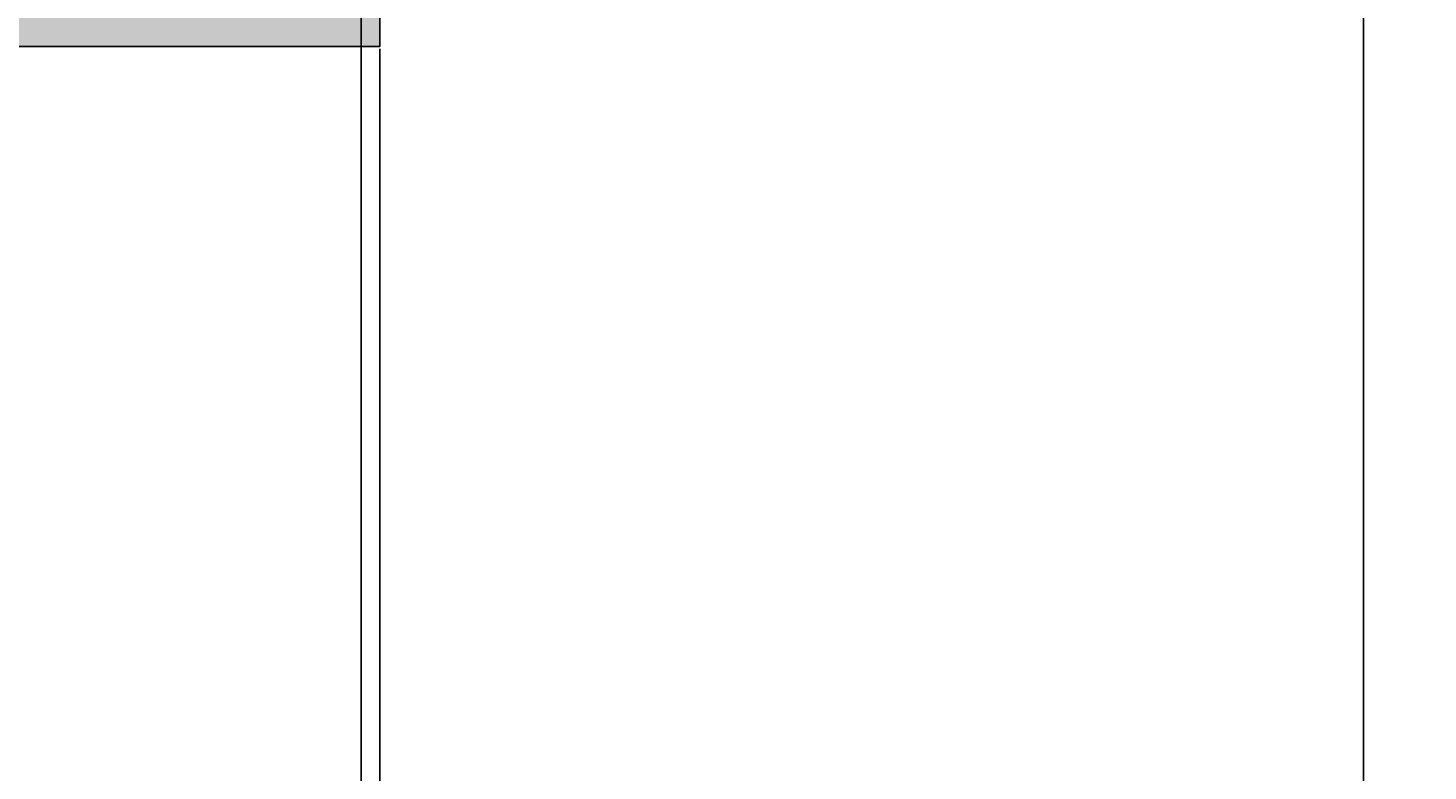
# Model space of a CAD drawing. Units: millimetres. Extents: x -11 to 280, y -4 to 208.
# Tile 40 of 55: x 222 to 262, y 85 to 106. Entities that reach past the tile are written whole.
import ezdxf

# ---------------------------------------------------------------- set-up
doc = ezdxf.new("R2010")
doc.units = ezdxf.units.MM
doc.layers.add('M-DIMS', color=2, linetype='Continuous', lineweight=18)
doc.layers.add('M-HYDR-PRES', color=7, linetype='Continuous', lineweight=25)
doc.layers.add('M-HYDR-PRES-PATT', color=240, linetype='Continuous', lineweight=13, true_color=0xed1f24)
doc.styles.get("Standard").update_dxf_attribs({"font": 'arial.ttf'})
doc.dimstyles.get("Standard").update_dxf_attribs({"dimtxt": 0.18, "dimasz": 0.18, "dimexe": 0.18, "dimexo": 0.0625, "dimgap": 0.09, "dimtad": 0, "dimtih": 1, "dimtoh": 1, "dimdec": 4, "dimzin": 0, "dimdsep": 46, "dimtxsty": 'Standard', "dimcen": 0.09, "dimadec": 0, "dimazin": 0, "dimtfac": 1, "dimtdec": 4, "dimtofl": 0, "dimtmove": 0, "dimatfit": 3, "dimfxl": 1, "dimtolj": 1, "dimtzin": 0, "dimarcsym": 0})

# ---------------------------------------------------------------- blocks, each defined once
blk = doc.blocks.new('*D5')
at = {"layer": 'Defpoints', "color": 0, "transparency": 16777216}
for p in [(24.759, 192.645), (-10.087, 11.435), (261.686, 11.435)]:
    blk.add_point(p, dxfattribs=at)
at = {"layer": 'M-DIMS', "color": 0, "lineweight": -2, "transparency": 16777216}
for p, q in [((24.696, 192.645), (-10.267, 192.645)), ((-10.087, 192.465), (-10.087, 102.222)), ((-10.087, 11.615), (-10.087, 101.858)), ((261.624, 11.435), (-10.267, 11.435))]:
    blk.add_line(p, q, dxfattribs=at)
at = {"layer": 'M-DIMS', "color": 0, "transparency": 16777216}
for points in [[(-10.117, 192.465), (-10.057, 192.465), (-10.087, 192.645)], [(-10.117, 11.615), (-10.057, 11.615), (-10.087, 11.435)]]:
    blk.add_solid(points, dxfattribs=at)
at = {"layer": 'M-DIMS', "color": 0, "transparency": 16777216, "insert": (-10.087, 102.04), "char_height": 0.18, "attachment_point": 5}
blk.add_mtext('\\A1;181.2', dxfattribs=at)
blk = doc.blocks.new('*D13')
at = {"layer": 'Defpoints', "color": 0, "transparency": 16777216}
for p in [(191.774, 105.314), (232.2, 105.314), (232.2, -3.415)]:
    blk.add_point(p, dxfattribs=at)
at = {"layer": 'M-DIMS', "color": 0, "lineweight": -2, "transparency": 16777216}
for p, q in [((191.774, 105.252), (191.774, -3.595)), ((232.2, 105.252), (232.2, -3.595)), ((191.954, -3.415), (211.52, -3.415)), ((232.02, -3.415), (212.454, -3.415))]:
    blk.add_line(p, q, dxfattribs=at)
at = {"layer": 'M-DIMS', "color": 0, "transparency": 16777216}
for points in [[(191.954, -3.385), (191.954, -3.445), (191.774, -3.415)], [(232.02, -3.385), (232.02, -3.445), (232.2, -3.415)]]:
    blk.add_solid(points, dxfattribs=at)
at = {"layer": 'M-DIMS', "color": 0, "transparency": 16777216, "insert": (211.987, -3.415), "char_height": 0.18, "attachment_point": 5}
blk.add_mtext('\\A1;40.426', dxfattribs=at)
blk = doc.blocks.new('*D20')
at = {"layer": 'Defpoints', "color": 0, "transparency": 16777216}
for p in [(231.68, 207.495), (151.022, 43.599), (231.68, 43.599)]:
    blk.add_point(p, dxfattribs=at)
at = {"layer": 'M-DIMS', "color": 0, "lineweight": -2, "transparency": 16777216}
for p, q in [((151.022, 43.662), (151.022, 207.675)), ((231.68, 43.662), (231.68, 207.675)), ((151.202, 207.495), (190.957, 207.495)), ((231.5, 207.495), (191.745, 207.495))]:
    blk.add_line(p, q, dxfattribs=at)
at = {"layer": 'M-DIMS', "color": 0, "transparency": 16777216}
for points in [[(151.202, 207.525), (151.202, 207.465), (151.022, 207.495)], [(231.5, 207.525), (231.5, 207.465), (231.68, 207.495)]]:
    blk.add_solid(points, dxfattribs=at)
at = {"layer": 'M-DIMS', "color": 0, "transparency": 16777216, "insert": (191.351, 207.495), "char_height": 0.18, "attachment_point": 5}
blk.add_mtext('\\A1;80.66', dxfattribs=at)
blk = doc.blocks.new('*D22')
at = {"layer": 'Defpoints', "color": 0, "transparency": 16777216}
for p in [(259.871, 207.495), (231.68, 34.723), (259.871, 34.723)]:
    blk.add_point(p, dxfattribs=at)
at = {"layer": 'M-DIMS', "color": 0, "lineweight": -2, "transparency": 16777216}
for p, q in [((231.68, 34.785), (231.68, 207.675)), ((259.871, 34.785), (259.871, 207.675)), ((231.86, 207.495), (245.38, 207.495)), ((259.691, 207.495), (246.171, 207.495))]:
    blk.add_line(p, q, dxfattribs=at)
at = {"layer": 'M-DIMS', "color": 0, "transparency": 16777216}
for points in [[(231.86, 207.525), (231.86, 207.465), (231.68, 207.495)], [(259.691, 207.525), (259.691, 207.465), (259.871, 207.495)]]:
    blk.add_solid(points, dxfattribs=at)
at = {"layer": 'M-DIMS', "color": 0, "transparency": 16777216, "insert": (245.776, 207.495), "char_height": 0.18, "attachment_point": 5}
blk.add_mtext('\\A1;28.19', dxfattribs=at)

msp = doc.modelspace()

# ---------------------------------------------------------------- hatches: boundary and pattern name
at = {"layer": 'M-HYDR-PRES-PATT'}
h = msp.add_hatch(color=256, dxfattribs=at)
h.set_gradient(color1=(237, 31, 36), color2=(237, 31, 36), tint=1)
h.paths.add_polyline_path([(232.2, 133.1228), (228.7, 133.1228), (228.7, 108.8141), (102.7646, 108.8141), (102.7646, 105.3141), (232.2, 105.3141)])
h.paths.add_polyline_path([(128.8433, 105.3141), (125.3433, 105.3141), (125.3433, 91.7099, 1), (128.8433, 91.7099)])
h.paths.add_polyline_path([(229.1617, 78.7098), (196.7745, 78.7098, -0.4142136), (191.7745, 83.7098), (191.7745, 105.3141), (188.2745, 105.3141), (188.2745, 80.2098, 0.4142136), (193.2745, 75.2098), (225.6617, 75.2098), (225.6617, 43.5991), (229.1617, 43.5991)])
h.paths.add_polyline_path([(102.7646, 110.3704), (95.5776, 110.3704), (95.5776, 103.9022), (102.7646, 103.9022)])
h.paths.add_polyline_path([(100.7059, 107.2502), (99.1711, 106.3641), (99.1711, 106.8641), (97.1711, 106.8641), (97.1711, 107.6363), (99.1711, 107.6363), (99.1711, 108.1363)], flags=16)
h.paths.add_polyline_path([(234.6119, 138.4081), (226.5106, 138.4081), (226.5106, 133.1228), (234.6119, 133.1228)])
h.paths.add_polyline_path([(231.1963, 135.7055), (230.2965, 134.1786), (229.4241, 135.7213), (229.9241, 135.7168), (229.9418, 137.7167), (230.7141, 137.7099), (230.6963, 135.71)], flags=16)

# ---------------------------------------------------------------- linework, layer by layer
at = {"layer": 'M-HYDR-PRES'}
msp.add_lwpolyline([(232.2, 133.1228), (232.2, 105.3141), (102.7646, 105.3141)], dxfattribs=at)

# ---------------------------------------------------------------- dimensions: what is measured, and where the dimension line sits
at = {"layer": 'M-DIMS'}
for base, p1, p2, override, picture, middle in [((231.6803, 207.495), (151.0217, 43.5991), (231.6803, 43.5991), {"dimdec": 2, "dimlfac": 1, "dimrnd": 0, "dimzin": 0, "dimdsep": 46, "dimlunit": 2}, '*D20', (191.351, 207.495)), ((259.871, 207.495), (231.6803, 34.7226), (259.871, 34.7226), {"dimdec": 2, "dimlfac": 1, "dimrnd": 0, "dimzin": 0, "dimdsep": 46, "dimlunit": 2}, '*D22', (245.7757, 207.495)), ((232.20002, -3.41542), (191.77448, 105.31407), (232.20002, 105.31407), {"dimdec": 3, "dimlfac": 1, "dimrnd": 0, "dimzin": 0, "dimdsep": 46, "dimlunit": 2}, '*D13', (211.98725, -3.41542))]:
    dim = msp.add_linear_dim(base=base, p1=p1, p2=p2, dimstyle='Standard', override=override, dxfattribs=at)
    dim.commit()
    dim.dimension.update_dxf_attribs({"geometry": picture, "text_midpoint": middle})
dim = msp.add_linear_dim(base=(-10.0865, 11.4346), p1=(24.7588, 192.645), p2=(261.6863, 11.4346), angle=90, dimstyle='Standard', override={"dimdec": 1, "dimlfac": 1, "dimrnd": 0, "dimzin": 0, "dimdsep": 46, "dimlunit": 2}, dxfattribs=at)
dim.commit()
dim.dimension.update_dxf_attribs({"geometry": '*D5', "text_midpoint": (-10.0865, 102.0398)})

doc.saveas('drawing.dxf')
